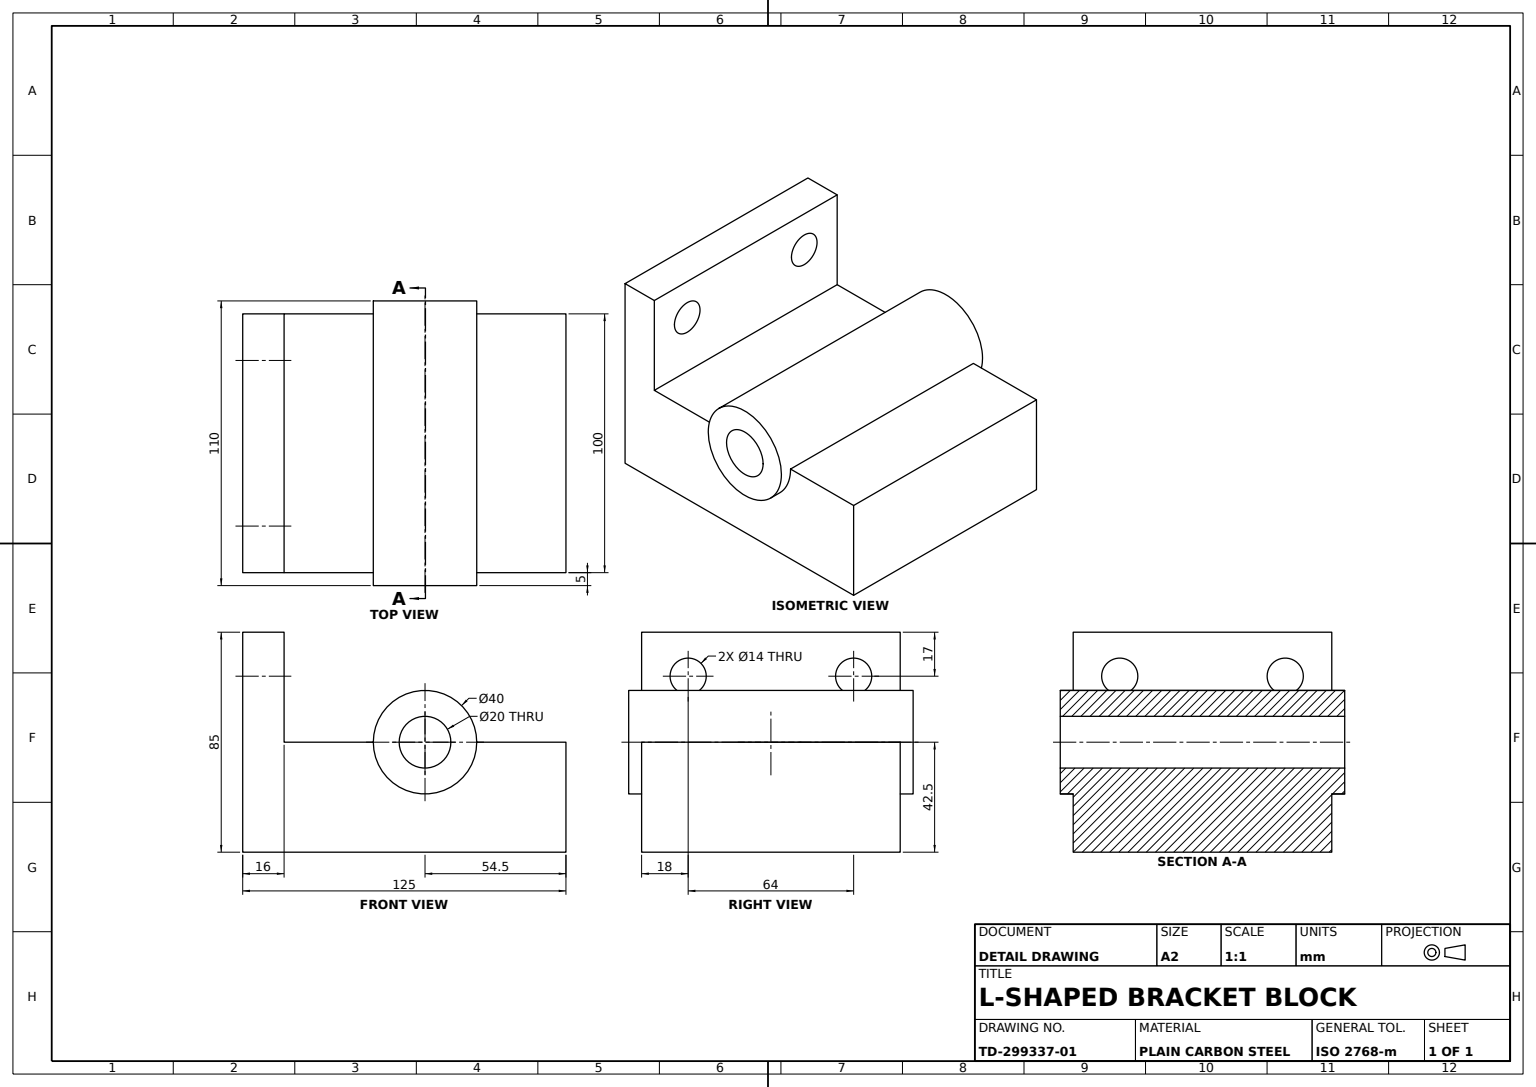
from build123d import *

# Parameters (mm, degrees)
L_BRACKET_BODY_DEPTH           = 100
MOUNTING_HOLES_SKETCH_R        = 7
MOUNTING_HOLES_2X_14_DEPTH     = 100
TRUNNION_SKETCH_R              = 20
TRUNNION_40_DEPTH              = 100
TRUNNION_START                 = 5
TRUNNION_END_BOSS_A_SKETCH_R   = 20
TRUNNION_END_BOSS_A_40X5_DEPTH = 5
TRUNNION_END_BOSS_B_SKETCH_R   = 20
TRUNNION_END_BOSS_B_40X5_DEPTH = 5
TRUNNION_BORE_SKETCH_R         = 10
TRUNNION_BORE_20_DEPTH         = 110


with BuildPart() as part:
    # L Bracket Profile Sketch → L Bracket Body (new body)
    with BuildSketch(Plane.XY):
        Polygon((0, 0), (125, 0), (125, 42.5), (16, 42.5), (16, 85), (0, 85), align=None)
    extrude(amount=-L_BRACKET_BODY_DEPTH)

    # Mounting Holes Sketch → Mounting Holes 2xØ14 (cut)
    with BuildSketch(Plane(origin=(16, 0, 0), x_dir=(0, 0, -1), z_dir=(1, 0, 0))):
        with Locations((18, 68)):
            Circle(MOUNTING_HOLES_SKETCH_R)
        with Locations((82, 68)):
            Circle(MOUNTING_HOLES_SKETCH_R)
    extrude(amount=-MOUNTING_HOLES_2X_14_DEPTH, mode=Mode.SUBTRACT)

    # Trunnion Sketch → Trunnion Ø40 (add)
    with BuildSketch(Plane.XY):
        with Locations((70.5, 42.5)):
            Circle(TRUNNION_SKETCH_R)
    extrude(amount=-TRUNNION_40_DEPTH)

    # Trunnion End Boss A Sketch → Trunnion End Boss A Ø40x5 (add)
    with BuildSketch(Plane.XY.offset(TRUNNION_START)):
        with Locations((70.5, 42.5)):
            Circle(TRUNNION_END_BOSS_A_SKETCH_R)
    extrude(amount=-TRUNNION_END_BOSS_A_40X5_DEPTH)

    # Trunnion End Boss B Sketch → Trunnion End Boss B Ø40x5 (add)
    with BuildSketch(Plane(origin=(0, 0, -100), x_dir=(-1, 0, 0), z_dir=(0, 0, -1))):
        with Locations(Location((-70.5, 42.5, 0), (0, 0, 180))):
            Circle(TRUNNION_END_BOSS_B_SKETCH_R)
    extrude(amount=TRUNNION_END_BOSS_B_40X5_DEPTH)

    # Trunnion Bore Sketch → Trunnion Bore Ø20 (cut)
    with BuildSketch(Plane(origin=(0, 0, -105), x_dir=(-1, 0, 0), z_dir=(0, 0, -1))):
        with Locations((-70.5, 42.5)):
            Circle(TRUNNION_BORE_SKETCH_R)
    extrude(amount=-TRUNNION_BORE_20_DEPTH, mode=Mode.SUBTRACT)


solid = part.part
